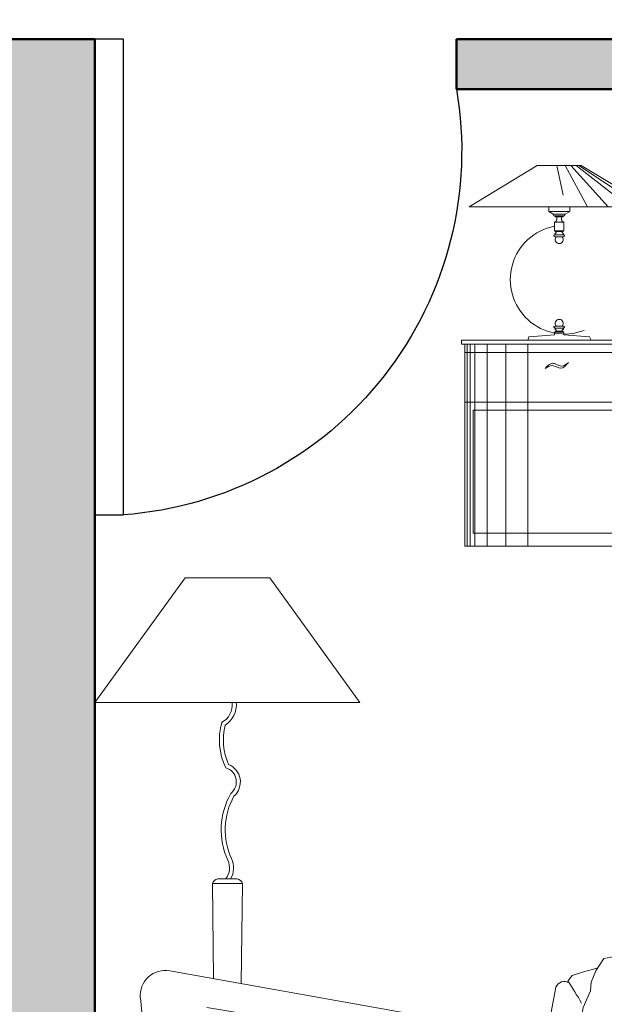
# Model space of a CAD drawing. Units: inches. Extents: x 1771 to 3025, y 319 to 889.
# Tile 27 of 35: x 2863 to 2921, y 521 to 619. Entities that reach past the tile are written whole.
import ezdxf

# ---------------------------------------------------------------- set-up
doc = ezdxf.new("R2010")
doc.units = ezdxf.units.IN
doc.header["$MEASUREMENT"] = 0
for name, color, linetype, lineweight in [('A-DOOR', 4, 'Continuous', 25), ('A-FURN', 8, 'Continuous', 18), ('A-WALL', 7, 'Continuous', 50), ('A-WALL-PATT', 254, 'Continuous', 13)]:
    doc.layers.add(name, color=color, linetype=linetype, lineweight=lineweight)

# ---------------------------------------------------------------- blocks, each defined once
blk = doc.blocks.new('A$C3908634B')
for p, q in [((184.3, 923.4), (19, 823.1)), ((237.5, 923.4), (184.3, 923.4)), ((190.2, 923.4), (237.5, 923.4)), ((231.9, 923.4), (247.3, 851.1)), ((284.7, 923.4), (237.5, 923.4)), ((237.5, 923.4), (290.6, 923.4)), ((251.7, 923.4), (305.7, 823.1)), ((266, 923.4), (356.4, 823.1)), ((278.7, 923.4), (406.8, 823.1)), ((284.7, 923.4), (436.3, 823.1)), ((290.6, 923.4), (456, 823.1)), ((237.5, 823.1), (19, 823.1)), ((212, 823.1), (212, 811.7)), ((237.5, 823.1), (456, 823.1)), ((263, 823.1), (263, 811.7)), ((212, 811.7), (223, 805.4)), ((212, 811.7), (237.5, 811.7)), ((223, 805.4), (224.6, 801.4)), ((223, 805.4), (237.5, 805.4)), ((250.4, 801.4), (224.6, 801.4)), ((226.9, 801.4), (228.3, 798.3)), ((228.3, 798.3), (237.5, 798.3)), ((228.3, 798.3), (231.3, 797.6)), ((231.1, 790.5), (230.2, 788)), ((231.5, 791.1), (231.1, 790.5)), ((231.3, 797.6), (232, 794.9)), ((231.6, 792.6), (231.5, 791.9)), ((231.5, 791.9), (231.5, 791.1)), ((231.9, 793.9), (231.6, 792.6)), ((232, 794.9), (231.9, 793.9)), ((263, 811.7), (237.5, 811.7)), ((252, 805.4), (237.5, 805.4)), ((246.7, 798.3), (237.5, 798.3)), ((243.7, 797.6), (243, 794.9)), ((243, 794.9), (243.1, 793.9)), ((243.1, 793.9), (243.4, 792.6)), ((243.4, 792.6), (243.4, 791.9)), ((243.4, 791.9), (243.4, 791.1)), ((243.4, 791.1), (243.9, 790.5)), ((246.7, 798.3), (243.7, 797.6)), ((243.9, 790.5), (244.8, 788)), ((248.1, 801.4), (246.7, 798.3)), ((252, 805.4), (250.4, 801.4)), ((263, 811.7), (252, 805.4)), ((227.8, 786.4), (226.2, 785.6)), ((226.2, 785.6), (226.2, 765)), ((226.2, 785.6), (248.8, 785.6)), ((226.2, 765), (227.6, 764.2)), ((226.2, 765), (237.5, 765)), ((227.6, 764.2), (228.5, 763.3)), ((230.2, 788), (227.8, 786.4)), ((248.8, 765), (237.5, 765)), ((244.8, 788), (247.2, 786.4)), ((247.4, 764.2), (246.5, 763.3)), ((247.2, 786.4), (248.8, 785.6)), ((248.8, 765), (247.4, 764.2)), ((248.8, 785.6), (248.8, 765)), ((224.8, 753.5), (224.7, 752.9)), ((224.7, 752.9), (224.8, 752.1)), ((225.3, 753.9), (224.8, 753.5)), ((224.8, 752.1), (225.2, 751.4)), ((225.2, 751.4), (225.6, 750.9)), ((225.7, 754.3), (225.3, 753.9)), ((225.6, 750.9), (228.1, 750.2)), ((226.3, 754.6), (225.7, 754.3)), ((227, 754.7), (226.3, 754.6)), ((227.9, 754.7), (227, 754.7)), ((227.4, 757.9), (227.1, 757.2)), ((227.1, 757.2), (227.3, 756.6)), ((227.3, 756.6), (227.8, 755.9)), ((227.7, 758.5), (227.4, 757.9)), ((228.6, 758.7), (227.7, 758.5)), ((227.8, 755.9), (228.9, 755.2)), ((228.9, 755.2), (227.9, 754.7)), ((228.1, 750.2), (229.9, 750)), ((228.5, 763.3), (229.4, 762.5)), ((228.5, 763.3), (237.5, 763.3)), ((229.4, 759.1), (228.6, 758.7)), ((228.9, 755.2), (237.5, 755.2)), ((229.4, 762.5), (230, 761.4)), ((229.8, 759.5), (229.4, 759.1)), ((230.1, 760.2), (229.8, 759.5)), ((229.9, 750), (232.4, 750.2)), ((230, 761.4), (230.1, 760.2)), ((232.4, 750.2), (237.5, 750.2)), ((246.5, 763.3), (237.5, 763.3)), ((246.1, 755.2), (237.5, 755.2)), ((242.6, 750.2), (237.5, 750.2)), ((245.1, 750), (242.6, 750.2)), ((245, 761.4), (244.9, 760.2)), ((244.9, 760.2), (245.2, 759.5)), ((245.6, 762.5), (245, 761.4)), ((246.9, 750.2), (245.1, 750)), ((245.2, 759.5), (245.6, 759.1)), ((246.5, 763.3), (245.6, 762.5)), ((245.6, 759.1), (246.4, 758.7)), ((247.2, 755.9), (246.1, 755.2)), ((246.1, 755.2), (247.1, 754.7)), ((246.4, 758.7), (247.3, 758.5)), ((249.4, 750.9), (246.9, 750.2)), ((247.1, 754.7), (248, 754.7)), ((247.7, 756.6), (247.2, 755.9)), ((247.3, 758.5), (247.6, 757.9)), ((247.6, 757.9), (247.9, 757.2)), ((247.9, 757.2), (247.7, 756.6)), ((248, 754.7), (248.7, 754.6)), ((248.7, 754.6), (249.3, 754.3)), ((249.3, 754.3), (249.7, 753.9)), ((249.8, 751.4), (249.4, 750.9)), ((249.7, 753.9), (250.2, 753.5)), ((250.2, 752.1), (249.8, 751.4)), ((250.2, 753.5), (250.3, 752.9)), ((250.3, 752.9), (250.2, 752.1)), ((224.7, 530.9), (224.8, 531.7)), ((224.8, 530.3), (224.7, 530.9)), ((224.8, 531.7), (225.2, 532.4)), ((225.3, 529.9), (224.8, 530.3)), ((225.2, 532.4), (225.6, 532.9)), ((225.7, 529.5), (225.3, 529.9)), ((225.6, 532.9), (228.1, 533.6)), ((226.3, 529.2), (225.7, 529.5)), ((227, 529.1), (226.3, 529.2)), ((227.9, 529.1), (227, 529.1)), ((227.1, 526.6), (227.3, 527.2)), ((227.4, 525.9), (227.1, 526.6)), ((227.3, 527.2), (227.8, 527.9)), ((227.7, 525.3), (227.4, 525.9)), ((228.6, 525.1), (227.7, 525.3)), ((227.8, 527.9), (228.9, 528.6)), ((228.9, 528.6), (227.9, 529.1)), ((228.1, 533.6), (229.9, 533.8)), ((228.9, 528.6), (237.5, 528.6)), ((230.3, 533.8), (237.5, 533.6)), ((242.6, 533.6), (237.5, 533.6)), ((246.1, 528.6), (237.5, 528.6)), ((245.1, 533.8), (242.6, 533.6)), ((246.9, 533.6), (245.1, 533.8)), ((246.1, 528.6), (247.1, 529.1)), ((247.2, 527.9), (246.1, 528.6)), ((246.4, 525.1), (247.3, 525.3)), ((249.4, 532.9), (246.9, 533.6)), ((247.1, 529.1), (248, 529.1)), ((247.7, 527.2), (247.2, 527.9)), ((247.3, 525.3), (247.6, 525.9)), ((247.6, 525.9), (247.9, 526.6)), ((247.9, 526.6), (247.7, 527.2)), ((248, 529.1), (248.7, 529.2)), ((248.7, 529.2), (249.3, 529.5)), ((249.3, 529.5), (249.7, 529.9)), ((249.8, 532.4), (249.4, 532.9)), ((249.7, 529.9), (250.2, 530.3)), ((250.2, 531.7), (249.8, 532.4)), ((250.3, 530.9), (250.2, 531.7)), ((250.2, 530.3), (250.3, 530.9)), ((164, 507.9), (161.1, 499.5)), ((164, 507.9), (226.2, 512.1)), ((226.2, 518.8), (227.6, 519.6)), ((226.2, 512.1), (226.2, 518.8)), ((226.2, 518.8), (237.5, 518.8)), ((227.6, 519.6), (228.5, 520.5)), ((228.5, 520.5), (229.4, 521.3)), ((229.4, 524.7), (228.6, 525.1)), ((229.8, 524.3), (229.4, 524.7)), ((229.4, 521.3), (230, 522.4)), ((229.4, 521.3), (237.5, 521.3)), ((230.1, 523.6), (229.8, 524.3)), ((230, 522.4), (230.1, 523.6)), ((245.6, 521.3), (237.5, 521.3)), ((248.8, 518.8), (237.5, 518.8)), ((244.9, 523.6), (245.2, 524.3)), ((245, 522.4), (244.9, 523.6)), ((245.6, 521.3), (245, 522.4)), ((245.2, 524.3), (245.6, 524.7)), ((245.6, 524.7), (246.4, 525.1)), ((246.5, 520.5), (245.6, 521.3)), ((247.4, 519.6), (246.5, 520.5)), ((248.8, 518.8), (247.4, 519.6)), ((248.8, 512.1), (248.8, 518.8)), ((311, 507.9), (248.8, 512.1)), ((311, 507.9), (315.3, 499.5)), ((475, 499.5), (0, 499.5)), ((0, 499.5), (0, 489.5)), ((475, 489.5), (0, 489.5)), ((8.7, 489.5), (8.7, 0)), ((14.1, 488.6), (14.1, 0)), ((21.3, 488.6), (21.3, 0)), ((33, 488.6), (33, 0)), ((62.7, 488.6), (62.7, 0)), ((107.6, 488.6), (107.6, 0)), ((161.1, 499.5), (237.5, 499.5)), ((161.6, 488.6), (161.6, 0)), ((315.3, 499.5), (237.5, 499.5)), ((467.1, 469.5), (8.7, 469.5)), ((467.1, 349.5), (8.7, 349.5)), ((28.7, 329.5), (28.7, 31.6)), ((447.1, 329.5), (28.7, 329.5)), ((28.7, 31.6), (447.1, 31.6)), ((8.7, 0), (467.1, 0))]:
    blk.add_line(p, q)
for centre, radius, start, end in [((250.5, 646.2), 131.8, 100.6234, 291.2), ((237.5, 743.5), 9.69, 137.7341, 270), ((237.5, 743.5), 9.69, 270, 42.2659), ((237.5, 540.3), 9.69, 90, 222.2659), ((237.5, 540.3), 9.69, 317.7341, 90)]:
    blk.add_arc(centre, radius, start, end)
for points, knots in [([(259.6, 445.5), (254.3, 441.1), (244.8, 433.2), (231.9, 440.9), (217, 446), (209.2, 437.1), (203.4, 430.5)], [0, 0, 0, 0, 18.381528, 32.980054, 40.875646, 63.595153, 63.595153, 63.595153, 63.595153]), ([(259.6, 445.5), (254, 438.6), (242.8, 424.9), (221, 442.9), (208.9, 434.4), (203.4, 430.5)], [0, 0, 0, 0, 22.772447, 45.052082, 63.466582, 63.466582, 63.466582, 63.466582])]:
    blk.add_open_spline(points, degree=3, knots=knots)
blk = doc.blocks.new('A$C0DCF6C46')
for p, q in [((179.4, 1650), (0, 1402.3)), ((179.4, 1650), (0, 1402.3)), ((179.4, 1650), (347.3, 1650)), ((179.4, 1650), (347.3, 1650)), ((347.3, 1650), (526.7, 1402.3)), ((347.3, 1650), (526.7, 1402.3)), ((0, 1402.3), (526.7, 1402.3)), ((0, 1402.3), (526.7, 1402.3)), ((1202.6, 1072.4), (1213.4, 1083.3)), ((1202.6, 1072.4), (1213.4, 1083.3)), ((1213.4, 1083.3), (1227.6, 1090.4)), ((1213.4, 1083.3), (1227.6, 1090.4)), ((1227.6, 1090.4), (1251, 1095.4)), ((1227.6, 1090.4), (1251, 1095.4)), ((1251, 1095.4), (1277.5, 1092)), ((1251, 1095.4), (1277.5, 1092)), ((1277.5, 1092), (1301.8, 1082.8)), ((1277.5, 1092), (1301.8, 1082.8)), ((1301.8, 1082.8), (1321.9, 1067.8)), ((1301.8, 1082.8), (1321.9, 1067.8)), ((1173.6, 1032.9), (1189.7, 1057.2)), ((1173.6, 1032.9), (1189.7, 1057.2)), ((1189.7, 1057.2), (1202.6, 1072.4)), ((1189.7, 1057.2), (1202.6, 1072.4)), ((1259.7, 1050.3), (1237.5, 1065.3)), ((1259.7, 1050.3), (1237.5, 1065.3)), ((1321.9, 1067.8), (1345.5, 1041.1)), ((1321.9, 1067.8), (1345.5, 1041.1)), ((233.4, 1042.3), (293.3, 1042.3)), ((233.4, 1042.3), (235.7, 853.7)), ((233.4, 1042.3), (293.3, 1042.3)), ((233.4, 1042.3), (235.7, 853.7)), ((244, 1051.7), (282.6, 1051.7)), ((244, 1051.7), (282.6, 1051.7)), ((293.3, 1042.3), (290.8, 843.9)), ((293.3, 1042.3), (290.8, 843.9)), ((1255.9, 1046.6), (1245.7, 1027.6)), ((1255.9, 1046.6), (1245.7, 1027.6)), ((1278.7, 1041.6), (1259.7, 1050.3)), ((1278.7, 1041.6), (1259.7, 1050.3)), ((1308.3, 1028.1), (1278.7, 1041.6)), ((1308.3, 1028.1), (1278.7, 1041.6)), ((1345.5, 1041.1), (1350.1, 1013.5)), ((1345.5, 1041.1), (1350.1, 1013.5)), ((1150.8, 970.5), (1173.6, 1032.9)), ((1150.8, 970.5), (1173.6, 1032.9)), ((1245.7, 1027.6), (1232.3, 1009.1)), ((1245.7, 1027.6), (1232.3, 1009.1)), ((1335.8, 1012.5), (1308.3, 1028.1)), ((1335.8, 1012.5), (1308.3, 1028.1)), ((1232.3, 1009.1), (1218.3, 983.7)), ((1232.3, 1009.1), (1218.3, 983.7)), ((1338.8, 997.1), (1335.8, 1012.5)), ((1338.8, 997.1), (1335.8, 1012.5)), ((1350.1, 1013.5), (1354.2, 991.7)), ((1350.1, 1013.5), (1354.2, 991.7)), ((1190.8, 987.7), (1188, 972.3)), ((1190.8, 987.7), (1188, 972.3)), ((1202.9, 975.4), (1190.8, 987.7)), ((1202.9, 975.4), (1190.8, 987.7)), ((1218.3, 983.7), (1202.9, 975.4)), ((1218.3, 983.7), (1202.9, 975.4)), ((1277.8, 994.4), (1265.6, 995)), ((1277.8, 994.4), (1265.6, 995)), ((1266, 980.7), (1284.6, 977.9)), ((1266, 980.7), (1284.6, 977.9)), ((1291.5, 983.2), (1277.8, 994.4)), ((1291.5, 983.2), (1277.8, 994.4)), ((1333.4, 980.2), (1324.9, 973.9)), ((1333.4, 980.2), (1324.9, 973.9)), ((1354.2, 991.7), (1333.4, 980.2)), ((1354.2, 991.7), (1333.4, 980.2)), ((1334, 990.3), (1338.8, 997.1)), ((1334, 990.3), (1338.8, 997.1)), ((1147.4, 942.9), (1150.8, 970.5)), ((1147.4, 942.9), (1150.8, 970.5)), ((1188, 972.3), (1182.6, 958)), ((1188, 972.3), (1182.6, 958)), ((1304.1, 966.6), (1297.6, 940.6)), ((1304.1, 966.6), (1297.6, 940.6)), ((1309.5, 977.7), (1304.1, 966.6)), ((1309.5, 977.7), (1304.1, 966.6)), ((1309.4, 969), (1312.6, 964.7)), ((1314.7, 968.9), (1309.4, 969)), ((1309.4, 969), (1312.6, 964.7)), ((1314.7, 968.9), (1309.4, 969)), ((1317.5, 977.7), (1309.5, 977.7)), ((1317.5, 977.7), (1309.5, 977.7)), ((1322.1, 963.3), (1318.8, 948.5)), ((1322.1, 963.3), (1318.8, 948.5)), ((1324.9, 973.9), (1322.1, 963.3)), ((1324.9, 973.9), (1322.1, 963.3)), ((1135.7, 928.2), (1147.4, 942.9)), ((1135.7, 928.2), (1147.4, 942.9)), ((1297.6, 940.6), (1286.8, 941.4)), ((1297.6, 940.6), (1286.8, 941.4)), ((1318.8, 948.5), (1307.6, 932.1)), ((1318.8, 948.5), (1307.6, 932.1)), ((1087.8, 908.4), (1135.7, 928.2)), ((1087.8, 908.4), (1135.7, 928.2)), ((1117, 920.9), (1113.7, 907.1)), ((1117, 920.9), (1113.7, 907.1)), ((1170.4, 917.1), (1156.8, 933.1)), ((1170.4, 917.1), (1156.8, 933.1)), ((1307.6, 932.1), (1282.5, 914.8)), ((1307.6, 932.1), (1282.5, 914.8)), ((1033.6, 897.7), (1060.7, 904.4)), ((1033.6, 897.7), (1060.7, 904.4)), ((1060.7, 904.4), (1087.8, 908.4)), ((1060.7, 904.4), (1087.8, 908.4)), ((1113.7, 907.1), (1121.7, 900.7)), ((1113.7, 907.1), (1121.7, 900.7)), ((1121.7, 900.7), (1119.4, 884.3)), ((1121.7, 900.7), (1119.4, 884.3)), ((1190.9, 864.1), (1144, 915.9)), ((1190.9, 864.1), (1144, 915.9)), ((1211.2, 886.7), (1170.4, 917.1)), ((1211.2, 886.7), (1170.4, 917.1)), ((1225.9, 897.6), (1208.3, 912.3)), ((1225.9, 897.6), (1208.3, 912.3)), ((1282.5, 914.8), (1267, 899.5)), ((1282.5, 914.8), (1267, 899.5)), ((1271.7, 895.8), (1295.1, 904.1)), ((1271.7, 895.8), (1295.1, 904.1)), ((1295.1, 904.1), (1310, 911.9)), ((1295.1, 904.1), (1310, 911.9)), ((1310, 911.9), (1334.4, 909.6)), ((1310, 911.9), (1334.4, 909.6)), ((1334.4, 909.6), (1359.2, 894.6)), ((1334.4, 909.6), (1359.2, 894.6)), ((995.7, 868.8), (1011.8, 893.6)), ((995.7, 868.8), (1011.8, 893.6)), ((1011.8, 893.6), (1033.6, 897.7)), ((1011.8, 893.6), (1033.6, 897.7)), ((1039.9, 891.8), (1050.5, 891.7)), ((1039.9, 891.8), (1050.5, 891.7)), ((1050.5, 891.7), (1058.4, 882.1)), ((1050.5, 891.7), (1058.4, 882.1)), ((1058.4, 882.1), (1076.1, 842.2)), ((1058.4, 882.1), (1076.1, 842.2)), ((1119.4, 884.3), (1119.3, 867.8)), ((1119.4, 884.3), (1119.3, 867.8)), ((1211.2, 886.7), (1190.9, 864.1)), ((1211.2, 886.7), (1190.9, 864.1)), ((1222.8, 881.9), (1223.6, 853.9)), ((1247, 848.8), (1222.8, 881.9)), ((1222.8, 881.9), (1223.6, 853.9)), ((1247, 848.8), (1222.8, 881.9)), ((1240.6, 890.8), (1225.9, 897.6)), ((1240.6, 890.8), (1225.9, 897.6)), ((1254.3, 890.2), (1240.6, 890.8)), ((1254.3, 890.2), (1240.6, 890.8)), ((1264.4, 895.9), (1254.3, 890.2)), ((1264.4, 895.9), (1254.3, 890.2)), ((1267, 899.5), (1271.7, 895.8)), ((1267, 899.5), (1271.7, 895.8)), ((1359.2, 894.6), (1384, 866.8)), ((1359.2, 894.6), (1384, 866.8)), ((148.7, 869.2), (799.3, 753.3)), ((148.7, 869.2), (799.3, 753.3)), ((986.5, 846.6), (995.7, 868.8)), ((986.5, 846.6), (995.7, 868.8)), ((1119.3, 867.8), (1135.5, 846.5)), ((1119.3, 867.8), (1135.5, 846.5)), ((1196.7, 865.6), (1204.6, 855)), ((1196.7, 865.6), (1204.6, 855)), ((1275.8, 869.8), (1284.7, 863.3)), ((1275.8, 869.8), (1284.7, 863.3)), ((1278.8, 848), (1280, 865.5)), ((1278.8, 848), (1280, 865.5)), ((1284.7, 863.3), (1296.3, 854.2)), ((1284.7, 863.3), (1296.3, 854.2)), ((1296.3, 854.2), (1303.8, 861.6)), ((1296.3, 854.2), (1303.8, 861.6)), ((1303.8, 861.6), (1313.5, 875.8)), ((1303.8, 861.6), (1313.5, 875.8)), ((1313.5, 875.8), (1318.8, 876.9)), ((1313.5, 875.8), (1318.8, 876.9)), ((1318.8, 876.9), (1321.4, 867.3)), ((1318.8, 876.9), (1321.4, 867.3)), ((1321.4, 867.3), (1342.5, 854.4)), ((1321.4, 867.3), (1342.5, 854.4)), ((1384, 866.8), (1396.6, 853.4)), ((1384, 866.8), (1396.6, 853.4)), ((984.8, 829.6), (986.5, 846.6)), ((984.8, 829.6), (986.5, 846.6)), ((1076.1, 842.2), (1077.8, 785.9)), ((1076.1, 842.2), (1077.8, 785.9)), ((1135.5, 846.5), (1162.3, 812.3)), ((1135.5, 846.5), (1162.3, 812.3)), ((1186.6, 860.4), (1212.2, 811.9)), ((1186.6, 860.4), (1212.2, 811.9)), ((1204.6, 855), (1219.4, 853.2)), ((1204.6, 855), (1219.4, 853.2)), ((1213.6, 851.7), (1221.1, 799.1)), ((1213.6, 851.7), (1221.1, 799.1)), ((1223.6, 853.9), (1255.4, 801.3)), ((1223.6, 853.9), (1255.4, 801.3)), ((1257.2, 799.9), (1247, 848.8)), ((1257.2, 799.9), (1247, 848.8)), ((1293.6, 844.7), (1278.8, 848)), ((1293.6, 844.7), (1278.8, 848)), ((1293.9, 818.2), (1293.6, 844.7)), ((1293.9, 818.2), (1293.6, 844.7)), ((1325.9, 840.7), (1312.2, 852)), ((1325.9, 840.7), (1312.2, 852)), ((1342.5, 854.4), (1362, 845.8)), ((1342.5, 854.4), (1362, 845.8)), ((1362, 845.8), (1365, 822.9)), ((1362, 845.8), (1365, 822.9)), ((1396.6, 853.4), (1411.8, 831)), ((1396.6, 853.4), (1411.8, 831)), ((1637.6, 846.8), (1643.1, 837.5)), ((1637.6, 846.8), (1643.1, 837.5)), ((915.2, 833), (897.4, 738.2)), ((915.2, 833), (897.4, 738.2)), ((970.2, 796.3), (984.8, 829.6)), ((970.2, 796.3), (984.8, 829.6)), ((1343.2, 816.2), (1325.9, 840.7)), ((1343.2, 816.2), (1325.9, 840.7)), ((1376.2, 822.8), (1365, 822.9)), ((1365, 822.9), (1371.3, 804.3)), ((1376.2, 822.8), (1365, 822.9)), ((1365, 822.9), (1371.3, 804.3)), ((1390.5, 825.9), (1376.2, 822.8)), ((1390.5, 825.9), (1376.2, 822.8)), ((1401.2, 832.2), (1390.5, 825.9)), ((1401.2, 832.2), (1390.5, 825.9)), ((1405.2, 808.3), (1401.2, 832.2)), ((1405.2, 808.3), (1401.2, 832.2)), ((1411.8, 831), (1422.3, 818.2)), ((1411.8, 831), (1422.3, 818.2)), ((1414.4, 832.1), (1447.5, 790.5)), ((1414.4, 832.1), (1447.5, 790.5)), ((1680.1, 723.7), (1660.3, 834.6)), ((1680.1, 723.7), (1660.3, 834.6)), ((167.7, 0), (90.2, 815.3)), ((167.7, 0), (90.2, 815.3)), ((1162.3, 812.3), (1187.5, 779.8)), ((1162.3, 812.3), (1187.5, 779.8)), ((1212.2, 811.9), (1236.7, 763.5)), ((1212.2, 811.9), (1236.7, 763.5)), ((1296.3, 781), (1293.9, 818.2)), ((1296.3, 781), (1293.9, 818.2)), ((1364.9, 799.6), (1343.2, 816.2)), ((1364.9, 799.6), (1343.2, 816.2)), ((1371.3, 804.3), (1380.5, 770.8)), ((1371.3, 804.3), (1380.5, 770.8)), ((1384, 803.7), (1372.4, 811.7)), ((1384, 803.7), (1372.4, 811.7)), ((1403.6, 803.5), (1384, 803.7)), ((1403.6, 803.5), (1384, 803.7)), ((1423.8, 807.1), (1403.6, 803.5)), ((1423.8, 807.1), (1403.6, 803.5)), ((1422.3, 818.2), (1423.8, 807.1)), ((1422.3, 818.2), (1423.8, 807.1)), ((821.8, 697.8), (222.3, 796.3)), ((821.8, 697.8), (222.3, 796.3)), ((966.3, 773.5), (970.2, 796.3)), ((966.3, 773.5), (970.2, 796.3)), ((1077.8, 785.9), (1071.1, 747.3)), ((1077.8, 785.9), (1071.1, 747.3)), ((1275.4, 760.5), (1257.2, 799.9)), ((1275.4, 760.5), (1257.2, 799.9)), ((1431.7, 801.7), (1440.8, 748.6)), ((1431.7, 801.7), (1440.8, 748.6)), ((1447.5, 790.5), (1463.6, 748.4)), ((1447.5, 790.5), (1463.6, 748.4)), ((963, 758.2), (966.3, 773.5)), ((963, 758.2), (966.3, 773.5)), ((1187.5, 779.8), (1212.2, 747.2)), ((1187.5, 779.8), (1212.2, 747.2)), ((1236.7, 763.5), (1253.3, 709.8)), ((1236.7, 763.5), (1253.3, 709.8)), ((1304.4, 731.6), (1296.3, 781)), ((1304.4, 731.6), (1296.3, 781)), ((1380.5, 770.8), (1387.2, 743.7)), ((1380.5, 770.8), (1387.2, 743.7)), ((965.8, 711), (963, 758.2)), ((965.8, 711), (963, 758.2)), ((1071.1, 747.3), (1070.3, 709.1)), ((1071.1, 747.3), (1070.3, 709.1)), ((1212.2, 747.2), (1239, 712)), ((1212.2, 747.2), (1239, 712)), ((1294.7, 714.7), (1275.4, 760.5)), ((1294.7, 714.7), (1275.4, 760.5)), ((1387.2, 743.7), (1387.1, 723)), ((1387.2, 743.7), (1387.1, 723)), ((1463.6, 748.4), (1467.1, 713.4)), ((1463.6, 748.4), (1467.1, 713.4)), ((816.5, 736.2), (823.2, 687.2)), ((816.5, 736.2), (823.2, 687.2)), ((1310.9, 687.6), (1304.4, 731.6)), ((1310.9, 687.6), (1304.4, 731.6)), ((949, 665.5), (965.8, 711)), ((949, 665.5), (965.8, 711)), ((1070.3, 709.1), (1067.4, 681)), ((1070.3, 709.1), (1067.4, 681)), ((1239, 712), (1250, 700.8)), ((1239, 712), (1250, 700.8)), ((1253.3, 709.8), (1262, 665.7)), ((1253.3, 709.8), (1262, 665.7)), ((1319.7, 657.3), (1294.7, 714.7)), ((1319.7, 657.3), (1294.7, 714.7)), ((1387.1, 723), (1385.3, 706.1)), ((1387.1, 723), (1385.3, 706.1)), ((1410.2, 693.1), (1433.6, 709.9)), ((1410.2, 693.1), (1433.6, 709.9)), ((1433.6, 709.9), (1459.6, 709.7)), ((1433.6, 709.9), (1459.6, 709.7)), ((1467.1, 713.4), (1510.5, 701.4)), ((1467.1, 713.4), (1510.5, 701.4)), ((823.2, 687.2), (840.7, 645.7)), ((823.2, 687.2), (840.7, 645.7)), ((919.8, 701.9), (919.8, 0)), ((919.8, 701.9), (919.8, 0)), ((1325.9, 701.8), (1321.2, 649.3)), ((1325.9, 701.8), (1321.2, 649.3)), ((1387.8, 675.8), (1325.9, 701.8)), ((1387.8, 675.8), (1325.9, 701.8)), ((1387.8, 675.8), (1410.2, 693.1)), ((1387.8, 675.8), (1410.2, 693.1)), ((1510.5, 701.4), (1562.3, 673.9)), ((1510.5, 701.4), (1562.3, 673.9)), ((1656.8, 701.9), (1656.8, 607.1)), ((1656.8, 701.9), (1656.8, 607.1)), ((816.1, 675.1), (831.6, 638.4)), ((816.1, 675.1), (831.6, 638.4)), ((952.4, 624.6), (949, 665.5)), ((952.4, 624.6), (949, 665.5)), ((968.1, 667.4), (995.8, 675.7)), ((968.1, 667.4), (995.8, 675.7)), ((995.8, 675.7), (1036.1, 673.3)), ((995.8, 675.7), (1036.1, 673.3)), ((1036.1, 673.3), (1074.2, 672.4)), ((1036.1, 673.3), (1074.2, 672.4)), ((1074.2, 672.4), (1099.7, 668.5)), ((1074.2, 672.4), (1099.7, 668.5)), ((1099.7, 668.5), (1130.9, 665.6)), ((1099.7, 668.5), (1130.9, 665.6)), ((1130.9, 665.6), (1156.4, 659.6)), ((1130.9, 665.6), (1156.4, 659.6)), ((1262, 665.7), (1274.2, 603)), ((1262, 665.7), (1274.2, 603)), ((1362.7, 657.4), (1387.8, 675.8)), ((1362.7, 657.4), (1387.8, 675.8)), ((1562.3, 673.9), (1616.6, 642.7)), ((1562.3, 673.9), (1616.6, 642.7)), ((840.7, 645.7), (862.6, 619.4)), ((840.7, 645.7), (862.6, 619.4)), ((1120.6, 625.4), (1130.3, 647.1)), ((1120.6, 625.4), (1130.3, 647.1)), ((1130.3, 647.1), (1138.8, 656.6)), ((1130.3, 647.1), (1138.8, 656.6)), ((1156.4, 659.6), (1194, 656.7)), ((1156.4, 659.6), (1194, 656.7)), ((1194, 656.7), (1230, 653.7)), ((1194, 656.7), (1230, 653.7)), ((1230, 653.7), (1248, 637.7)), ((1230, 653.7), (1248, 637.7)), ((1321.2, 649.3), (1340.1, 623.1)), ((1321.2, 649.3), (1340.1, 623.1)), ((1361.5, 647.4), (1329.7, 647.6)), ((1361.5, 647.4), (1329.7, 647.6)), ((1342.9, 632.7), (1362.7, 657.4)), ((1342.9, 632.7), (1362.7, 657.4)), ((1569.5, 644.7), (1548.9, 662.4)), ((1569.5, 644.7), (1548.9, 662.4)), ((831.6, 638.4), (853.4, 612.1)), ((831.6, 638.4), (853.4, 612.1)), ((1248, 637.7), (1261.6, 613.2)), ((1248, 637.7), (1261.6, 613.2)), ((1325.7, 613.7), (1342.9, 632.7)), ((1325.7, 613.7), (1342.9, 632.7)), ((1503.4, 603.8), (1505.1, 628.7)), ((1503.4, 603.8), (1505.1, 628.7)), ((1595.2, 618), (1569.5, 644.7)), ((1595.2, 618), (1569.5, 644.7)), ((1616.6, 642.7), (1655.6, 607.9)), ((1616.6, 642.7), (1655.6, 607.9)), ((853.4, 612.1), (858.7, 592.9)), ((853.4, 612.1), (858.7, 592.9)), ((862.6, 619.4), (867.8, 600.3)), ((862.6, 619.4), (867.8, 600.3)), ((961.2, 603.3), (952.4, 624.6)), ((961.2, 603.3), (952.4, 624.6)), ((1115.1, 607.9), (1115, 596.8)), ((1115.1, 607.9), (1115, 596.8)), ((1128.9, 611.5), (1115.1, 607.9)), ((1128.9, 611.5), (1115.1, 607.9)), ((1115.6, 599.4), (1119.9, 607.9)), ((1115.6, 599.4), (1119.9, 607.9)), ((1119.9, 607.9), (1120.6, 625.4)), ((1119.9, 607.9), (1120.6, 625.4)), ((1154.9, 605), (1128.9, 611.5)), ((1154.9, 605), (1128.9, 611.5)), ((1202.6, 606.7), (1154.9, 605)), ((1202.6, 606.7), (1154.9, 605)), ((1217.8, 581.7), (1202.6, 606.7)), ((1217.8, 581.7), (1202.6, 606.7)), ((1261.6, 613.2), (1259.1, 569.7)), ((1261.6, 613.2), (1259.1, 569.7)), ((1304.9, 592.7), (1325.7, 613.7)), ((1304.9, 592.7), (1325.7, 613.7)), ((1475.8, 608.8), (1478.2, 578)), ((1491.8, 546.1), (1475.8, 608.8)), ((1475.8, 608.8), (1478.2, 578)), ((1491.8, 546.1), (1475.8, 608.8)), ((1618.8, 582.8), (1595.2, 618)), ((1618.8, 582.8), (1595.2, 618)), ((1655.6, 607.9), (1695.2, 580.6)), ((1655.6, 607.9), (1695.2, 580.6)), ((867.8, 600.3), (810.7, 0)), ((867.8, 600.3), (810.7, 0)), ((858.7, 592.9), (816.6, 146.6)), ((858.7, 592.9), (816.6, 146.6)), ((994.1, 595.1), (961.2, 603.3)), ((994.1, 595.1), (961.2, 603.3)), ((1053.9, 576.6), (994.1, 595.1)), ((1053.9, 576.6), (994.1, 595.1)), ((1111.3, 595.2), (1113.2, 565.5)), ((1111.3, 595.2), (1113.2, 565.5)), ((1274.2, 603), (1280.6, 545.6)), ((1274.2, 603), (1280.6, 545.6)), ((1284.6, 575.8), (1304.9, 592.7)), ((1284.6, 575.8), (1304.9, 592.7)), ((1501, 578.9), (1503.4, 603.8)), ((1501, 578.9), (1503.4, 603.8)), ((1112.1, 561.3), (1053.9, 576.6)), ((1112.1, 561.3), (1053.9, 576.6)), ((1228.9, 581.6), (1217.8, 581.7)), ((1228.9, 581.6), (1217.8, 581.7)), ((1228.2, 558.8), (1228.9, 581.6)), ((1228.2, 558.8), (1228.9, 581.6)), ((1259.1, 569.7), (1252.7, 566)), ((1259.1, 569.7), (1252.7, 566)), ((1478.2, 578), (1493.9, 543.4)), ((1478.2, 578), (1493.9, 543.4)), ((1489.2, 562.6), (1501, 578.9)), ((1489.2, 562.6), (1501, 578.9)), ((1635.5, 547.1), (1618.8, 582.8)), ((1635.5, 547.1), (1618.8, 582.8)), ((1695.2, 580.6), (1732.1, 555.4)), ((1695.2, 580.6), (1732.1, 555.4)), ((1128.3, 528.3), (1112.1, 561.3)), ((1128.3, 528.3), (1112.1, 561.3)), ((1252.7, 566), (1228.2, 558.8)), ((1252.7, 566), (1228.2, 558.8)), ((1732.1, 555.4), (1753.8, 546.2)), ((1732.1, 555.4), (1753.8, 546.2)), ((1747.8, 525.5), (1746.4, 548.4)), ((1747.8, 525.5), (1746.4, 548.4)), ((1142.4, 502.7), (1128.3, 528.3)), ((1142.4, 502.7), (1128.3, 528.3)), ((1280.6, 545.6), (1294.5, 479.8)), ((1280.6, 545.6), (1294.5, 479.8)), ((1478.3, 517.6), (1491.8, 546.1)), ((1478.3, 517.6), (1491.8, 546.1)), ((1493.9, 543.4), (1527.3, 540.5)), ((1493.9, 543.4), (1527.3, 540.5)), ((1527.3, 540.5), (1578.2, 538)), ((1527.3, 540.5), (1578.2, 538)), ((1578.2, 538), (1610.5, 537.7)), ((1578.2, 538), (1610.5, 537.7)), ((1610.5, 537.7), (1634.4, 534.9)), ((1610.5, 537.7), (1634.4, 534.9)), ((1634.4, 534.9), (1652.2, 511.4)), ((1634.4, 534.9), (1652.2, 511.4)), ((1753.8, 546.2), (1776.6, 543.9)), ((1753.8, 546.2), (1776.6, 543.9)), ((1776.6, 543.9), (1784.6, 547)), ((1776.6, 543.9), (1784.6, 547)), ((1788.3, 543.8), (1777, 533.3)), ((1788.3, 543.8), (1777, 533.3)), ((1777, 533.3), (1777, 522.1)), ((1777, 533.3), (1777, 522.1)), ((1784.6, 547), (1807.3, 541.5)), ((1784.6, 547), (1807.3, 541.5)), ((1807.3, 541.5), (1836.4, 528.5)), ((1807.3, 541.5), (1836.4, 528.5)), ((1836.4, 528.5), (1857.6, 518.8)), ((1836.4, 528.5), (1857.6, 518.8)), ((1460.7, 501.8), (1478.3, 517.6)), ((1460.7, 501.8), (1478.3, 517.6)), ((1652.2, 511.4), (1671, 474.2)), ((1652.2, 511.4), (1671, 474.2)), ((1747.1, 502.7), (1747.8, 525.5)), ((1747.1, 502.7), (1747.8, 525.5)), ((1777, 522.1), (1776.8, 504.6)), ((1777, 522.1), (1776.8, 504.6)), ((1857.6, 518.8), (1884.1, 516)), ((1857.6, 518.8), (1884.1, 516)), ((1884.1, 516), (1912.1, 507.8)), ((1884.1, 516), (1912.1, 507.8)), ((1162.3, 464.9), (1142.4, 502.7)), ((1162.3, 464.9), (1142.4, 502.7)), ((1447.7, 477), (1460.7, 501.8)), ((1447.7, 477), (1460.7, 501.8)), ((1556.5, 478.8), (1575.3, 505.7)), ((1556.5, 478.8), (1575.3, 505.7)), ((1740, 481), (1747.1, 502.7)), ((1740, 481), (1747.1, 502.7)), ((1766.2, 498.3), (1749.2, 494.8)), ((1766.2, 498.3), (1749.2, 494.8)), ((1776.8, 504.6), (1766.2, 498.3)), ((1776.8, 504.6), (1766.2, 498.3)), ((1913, 492.4), (1906, 476.6)), ((1913, 492.4), (1906, 476.6)), ((1912.1, 507.8), (1913, 492.4)), ((1912.1, 507.8), (1913, 492.4)), ((1294.5, 479.8), (1303.6, 427.7)), ((1294.5, 479.8), (1303.6, 427.7)), ((1415.7, 451.8), (1447.7, 477)), ((1415.7, 451.8), (1447.7, 477)), ((1547.8, 455), (1556.5, 478.8)), ((1547.8, 455), (1556.5, 478.8)), ((1671, 474.2), (1681.4, 448.6)), ((1671, 474.2), (1681.4, 448.6)), ((1732.4, 458.3), (1740, 481)), ((1732.4, 458.3), (1740, 481)), ((1906, 476.6), (1884.1, 456)), ((1906, 476.6), (1884.1, 456)), ((1170.5, 433.5), (1162.3, 464.9)), ((1170.5, 433.5), (1162.3, 464.9)), ((1379, 432.4), (1415.7, 451.8)), ((1379, 432.4), (1415.7, 451.8)), ((1546.6, 431.1), (1547.8, 455)), ((1546.6, 431.1), (1547.8, 455)), ((1683.6, 450.7), (1697.6, 414)), ((1699.5, 448.5), (1683.6, 450.7)), ((1683.6, 450.7), (1697.6, 414)), ((1699.5, 448.5), (1683.6, 450.7)), ((1715.9, 452.6), (1699.5, 448.5)), ((1715.9, 452.6), (1699.5, 448.5)), ((1736.6, 455.1), (1715.9, 452.6)), ((1736.6, 455.1), (1715.9, 452.6)), ((1750.9, 447.5), (1736.6, 455.1)), ((1750.9, 447.5), (1736.6, 455.1)), ((1792.3, 453.6), (1780.1, 445.7)), ((1792.3, 453.6), (1780.1, 445.7)), ((1833.1, 442.1), (1792.3, 453.6)), ((1833.1, 442.1), (1792.3, 453.6)), ((1884.1, 456), (1859.1, 446.7)), ((1884.1, 456), (1859.1, 446.7)), ((1186.7, 397.9), (1170.5, 433.5)), ((1186.7, 397.9), (1170.5, 433.5)), ((1645.3, 444.1), (1649.7, 395.3)), ((1645.3, 444.1), (1649.7, 395.3)), ((1780.1, 445.7), (1750.9, 447.5)), ((1780.1, 445.7), (1750.9, 447.5)), ((1859.1, 446.7), (1833.1, 442.1)), ((1859.1, 446.7), (1833.1, 442.1)), ((862, 416.6), (851.4, 416.6)), ((862, 416.6), (851.4, 416.6)), ((1033.5, 416.6), (1544.9, 416.6)), ((1033.5, 416.6), (1544.9, 416.6)), ((1303.6, 427.7), (1308.2, 407)), ((1303.6, 427.7), (1308.2, 407)), ((1351.8, 416.7), (1315.1, 406.4)), ((1351.8, 416.7), (1315.1, 406.4)), ((1388.4, 423.3), (1351.8, 416.7)), ((1388.4, 423.3), (1351.8, 416.7)), ((1440.4, 418.1), (1388.4, 423.3)), ((1440.4, 418.1), (1388.4, 423.3)), ((1490.2, 415.6), (1440.4, 418.1)), ((1490.2, 415.6), (1440.4, 418.1)), ((1542.2, 420.5), (1490.2, 415.6)), ((1542.2, 420.5), (1490.2, 415.6)), ((1552.6, 389.1), (1542.2, 420.5)), ((1552.6, 389.1), (1542.2, 420.5)), ((1697.6, 414), (1703.2, 388)), ((1697.6, 414), (1703.2, 388)), ((882, 396.6), (866.1, 216.6)), ((882, 396.6), (866.1, 216.6)), ((1189.7, 380.9), (1186.7, 397.9)), ((1189.7, 380.9), (1186.7, 397.9)), ((1189.8, 391.5), (1189.7, 380.9)), ((1189.8, 391.5), (1189.7, 380.9)), ((1217.5, 406.6), (1189.8, 391.5)), ((1217.5, 406.6), (1189.8, 391.5)), ((1262, 404.2), (1217.5, 406.6)), ((1262, 404.2), (1217.5, 406.6)), ((1315.1, 406.4), (1262, 404.2)), ((1315.1, 406.4), (1262, 404.2)), ((1649.7, 395.3), (1660.1, 361.8)), ((1649.7, 395.3), (1660.1, 361.8)), ((1563, 357.2), (1552.6, 389.1)), ((1563, 357.2), (1552.6, 389.1)), ((1703.2, 388), (1711.8, 331.7)), ((1703.2, 388), (1711.8, 331.7)), ((1585.9, 307.2), (1563, 357.2)), ((1585.9, 307.2), (1563, 357.2)), ((1660.1, 361.8), (1662.9, 319.9)), ((1660.1, 361.8), (1662.9, 319.9)), ((1662.9, 319.9), (1645.5, 263.2)), ((1662.9, 319.9), (1645.5, 263.2)), ((1711.8, 331.7), (1721.8, 252.6)), ((1711.8, 331.7), (1721.8, 252.6)), ((1612.6, 261.4), (1585.9, 307.2)), ((1612.6, 261.4), (1585.9, 307.2)), ((1625.5, 214.1), (1612.6, 261.4)), ((1625.5, 214.1), (1612.6, 261.4)), ((1645.5, 263.2), (1632, 228.9)), ((1645.5, 263.2), (1632, 228.9)), ((1721.8, 252.6), (1729.7, 181.9)), ((1721.8, 252.6), (1729.7, 181.9)), ((846.1, 196.6), (829.9, 196.6)), ((846.1, 196.6), (829.9, 196.6)), ((1028.1, 196.6), (1544.2, 196.6)), ((1028.1, 196.6), (1544.2, 196.6)), ((1629.9, 164.2), (1625.5, 214.1)), ((1629.9, 164.2), (1625.5, 214.1)), ((1729.7, 181.9), (1734.7, 143.7)), ((1729.7, 181.9), (1734.7, 143.7)), ((825, 157.1), (152.8, 157.1)), ((825, 157.1), (152.8, 157.1)), ((989.7, 156.6), (1587.6, 156.6)), ((989.7, 156.6), (1587.6, 156.6)), ((1630.1, 127.6), (1629.9, 164.2)), ((1630.1, 127.6), (1629.9, 164.2)), ((825, 146.6), (153.8, 146.6)), ((825, 146.6), (153.8, 146.6)), ((243.8, 146.6), (221.9, 0)), ((243.8, 146.6), (221.9, 0)), ((244.6, 146.6), (245.3, 86.3)), ((244.6, 146.6), (245.3, 86.3)), ((282.1, 146.6), (281.3, 86.3)), ((282.1, 146.6), (281.3, 86.3)), ((746.4, 146.6), (768.4, 0)), ((746.4, 146.6), (768.4, 0)), ((989.7, 146.6), (1587.6, 146.6)), ((989.7, 146.6), (1587.6, 146.6)), ((1724.1, 142.7), (1698.1, 135)), ((1724.1, 142.7), (1698.1, 135)), ((1737.4, 151.1), (1724.1, 142.7)), ((1737.4, 151.1), (1724.1, 142.7)), ((1734.7, 143.7), (1737.8, 131)), ((1734.7, 143.7), (1737.8, 131)), ((1631, 102.1), (1630.1, 127.6)), ((1631, 102.1), (1630.1, 127.6)), ((1661.3, 116.7), (1650.2, 119.5)), ((1661.3, 116.7), (1650.2, 119.5)), ((1675.7, 123), (1661.3, 116.7)), ((1675.7, 123), (1661.3, 116.7)), ((1698.1, 135), (1675.7, 123)), ((1698.1, 135), (1675.7, 123)), ((1735.1, 122.5), (1717, 111.5)), ((1735.1, 122.5), (1717, 111.5)), ((1747.3, 126.1), (1735.1, 122.5)), ((1747.3, 126.1), (1735.1, 122.5)), ((1737.8, 131), (1747.9, 135.7)), ((1737.8, 131), (1747.9, 135.7)), ((1747.9, 135.7), (1755.6, 101.1)), ((1747.9, 135.7), (1755.6, 101.1)), ((236.8, 100), (245.2, 100)), ((236.8, 100), (245.2, 100)), ((1632.3, 70.8), (1631, 102.1)), ((1632.3, 70.8), (1631, 102.1)), ((1701, 106.3), (1675.6, 113.9)), ((1701, 106.3), (1675.6, 113.9)), ((1717, 111.5), (1701, 106.3)), ((1717, 111.5), (1701, 106.3)), ((1755.6, 101.1), (1777.7, 72.3)), ((1755.6, 101.1), (1777.7, 72.3)), ((234.6, 85), (244.2, 85)), ((234.6, 85), (244.2, 85)), ((245.3, 86.3), (281.3, 86.3)), ((245.3, 86.3), (281.3, 86.3)), ((239.8, 68.3), (239.8, 22.5)), ((239.8, 68.3), (286.9, 68.3)), ((239.8, 68.3), (239.8, 22.5)), ((239.8, 68.3), (286.9, 68.3)), ((286.9, 68.3), (286.9, 22.5)), ((286.9, 68.3), (286.9, 22.5)), ((1635.9, 52.2), (1632.3, 70.8)), ((1635.9, 52.2), (1632.3, 70.8)), ((1777.7, 72.3), (1806.8, 63.6)), ((1777.7, 72.3), (1806.8, 63.6)), ((1806.8, 63.6), (1841.7, 47.4)), ((1806.8, 63.6), (1841.7, 47.4)), ((1645.4, 43.1), (1635.9, 52.2)), ((1645.4, 43.1), (1635.9, 52.2)), ((1669.2, 38.7), (1645.4, 43.1)), ((1669.2, 38.7), (1645.4, 43.1)), ((1656.8, 41), (1656.8, 0)), ((1656.8, 41), (1656.8, 0)), ((1841.7, 47.4), (1849.6, 39.4)), ((1841.7, 47.4), (1849.6, 39.4)), ((1849.6, 39.4), (1849.4, 20.8)), ((1849.6, 39.4), (1849.4, 20.8)), ((116.8, 22.5), (116.8, 0)), ((116.8, 22.5), (165.6, 22.5)), ((116.8, 22.5), (116.8, 0)), ((116.8, 22.5), (165.6, 22.5)), ((225.2, 22.5), (409.9, 22.5)), ((225.2, 22.5), (409.9, 22.5)), ((409.9, 22.5), (409.9, 0)), ((409.9, 22.5), (409.9, 0)), ((1691.4, 35.3), (1669.2, 38.7)), ((1691.4, 35.3), (1669.2, 38.7)), ((1709, 35.2), (1691.4, 35.3)), ((1709, 35.2), (1691.4, 35.3)), ((1715.3, 26.6), (1709, 35.2)), ((1715.3, 26.6), (1709, 35.2)), ((1738, 13.7), (1715.3, 26.6)), ((1738, 13.7), (1715.3, 26.6)), ((1849.4, 20.8), (1824.4, 6.7)), ((1849.4, 20.8), (1824.4, 6.7)), ((1789.3, 2.7), (1738, 13.7)), ((1789.3, 2.7), (1738, 13.7)), ((1824.4, 6.7), (1789.3, 2.7)), ((1824.4, 6.7), (1789.3, 2.7)), ((116.8, 0), (409.9, 0)), ((116.8, 0), (409.9, 0)), ((919.8, 0), (937.1, 0)), ((919.8, 0), (937.1, 0)), ((1639.4, 0), (1656.8, 0)), ((1639.4, 0), (1656.8, 0))]:
    blk.add_line(p, q)
for centre, radius, start, end in [((232.2, 1398.2), 40.9, 298.591, 4.7801), ((232.2, 1398.2), 40.9, 298.591, 4.7801), ((232.2, 1398.2), 48.9, 302.7794, 4.7801), ((232.2, 1398.2), 48.9, 302.7794, 4.7801), ((374.6, 1328.2), 127.4, 164.5089, 205.7991), ((374.6, 1328.2), 127.4, 164.5089, 205.7991), ((374.6, 1328.2), 119.4, 166.0279, 204.234), ((374.6, 1328.2), 119.4, 166.0279, 204.234), ((251.6, 1244.5), 29.4, 308.7103, 73.8033), ((251.6, 1244.5), 29.4, 308.7103, 73.8033), ((251.6, 1244.5), 37.4, 311.1929, 67.9822), ((251.6, 1244.5), 37.4, 311.1929, 67.9822), ((395.6, 1149.4), 144.8, 150.115, 204.7751), ((395.6, 1149.4), 144.8, 150.115, 204.7751), ((395.6, 1149.4), 136.8, 150.7005, 204.7627), ((395.6, 1149.4), 136.8, 150.7005, 204.7627), ((231.9, 1073.6), 35.6, 321.9956, 25.2261), ((231.9, 1073.6), 35.6, 321.9956, 25.2261), ((231.9, 1073.6), 43.6, 329.6961, 25.182), ((231.9, 1073.6), 43.6, 329.6961, 25.182), ((246.1, 1038.6), 13.2, 98.8052, 163.9237), ((246.1, 1038.6), 13.2, 98.8052, 163.9237), ((280.6, 1038.6), 13.2, 16.0763, 81.1948), ((280.6, 1038.6), 13.2, 16.0763, 81.1948), ((1273.4, -169.1), 1079.2, 70.279, 86.636), ((1273.4, -169.1), 1079.2, 70.279, 86.636), ((139.9, 820), 50, 79.8912, 185.4337), ((139.9, 820), 50, 79.8912, 185.4337), ((1273.4, -169.1), 1079.2, 104.7019, 107.5271), ((1273.4, -169.1), 1079.2, 104.7019, 107.5271), ((933.1, 829.6), 18.2, 70.9411, 169.1012), ((933.1, 829.6), 18.2, 70.9411, 169.1012), ((1047.8, 778.9), 128.2, 140.7938, 148.0496), ((1047.8, 778.9), 128.2, 140.7938, 148.0496), ((241, 385.5), 838.8, 30.0042, 33.5227), ((241, 385.5), 838.8, 30.0042, 33.5227), ((2335, 385.5), 838.2, 146.5555, 159.4144), ((2335, 385.5), 838.2, 146.5555, 159.4144), ((1650.3, 825), 14.4, 42.1894, 120.2274), ((1650.3, 825), 14.4, 42.1894, 120.2274), ((796.6, 733.4), 20, 7.8584, 82.4843), ((796.6, 733.4), 20, 7.8584, 82.4843), ((929, 702.9), 43.5, 37.8135, 139.3209), ((929, 702.9), 43.5, 37.8135, 139.3209), ((1647.6, 702.9), 43.5, 45.0789, 176.3198), ((1647.6, 702.9), 43.5, 45.0789, 176.3198), ((923.6, 729.2), 27.6, 161.105, 262.178), ((923.6, 729.2), 27.6, 161.105, 262.178), ((929, 702.9), 33.5, 26.3854, 153.1276), ((929, 702.9), 33.5, 26.3854, 153.1276), ((1647.6, 702.9), 33.5, 26.8724, 191.3689), ((1647.6, 702.9), 33.5, 26.8724, 191.3689), ((1639.4, 689.8), 38.7, 155.7528, 188.1441), ((1639.4, 689.8), 38.7, 155.7528, 188.1441), ((1653, 729.2), 27.6, 277.822, 348.4179), ((1653, 729.2), 27.6, 277.822, 348.4179), ((2420.3, 406.7), 856.1, 160.2245, 163.3332), ((2420.3, 406.7), 856.1, 160.2245, 163.3332), ((2392.2, 407.9), 838, 160.7403, 162.7196), ((2392.2, 407.9), 838, 160.7403, 162.7196), ((156.3, 406.7), 856.1, 0.182, 12.766), ((156.3, 406.7), 856.1, 0.182, 12.766), ((176.7, 406.6), 845.7, 0.1617, 12.7147), ((176.7, 406.6), 845.7, 0.1617, 12.7147), ((241, 385.5), 838.8, 2.1238, 13.0913), ((241, 385.5), 838.8, 2.1238, 13.0913), ((862, 396.6), 20, 0, 90), ((862, 396.6), 20, 0, 90), ((1052.6, 376.5), 44.4, 115.3918, 154.207), ((1052.6, 376.5), 44.4, 115.3918, 154.207), ((178.3, 351), 836.1, 335.1756, 4.0003), ((178.3, 351), 836.1, 335.1756, 4.0003), ((2398.3, 351), 836.1, 179.4209, 204.8244), ((2398.3, 351), 836.1, 179.4209, 204.8244), ((846.1, 216.6), 20, 270, 0), ((846.1, 216.6), 20, 270, 0), ((1045.3, 237.5), 44.4, 202.0254, 247.0946), ((1045.3, 237.5), 44.4, 202.0254, 247.0946), ((1529.6, 238.5), 44.4, 289.1171, 341.8054), ((1529.6, 238.5), 44.4, 289.1171, 341.8054), ((262.7, 71.1), 23.1, 138.7741, 186.8798), ((262.7, 71.1), 23.1, 138.7741, 186.8798), ((263.9, 71.1), 23.1, 353.1202, 41.2259), ((263.9, 71.1), 23.1, 353.1202, 41.2259)]:
    blk.add_arc(centre, radius, start, end)
blk = doc.blocks.new('A$C4223307F')
blk.add_line((768.4, 0), (810.7, 0))
blk.add_blockref('A$C0DCF6C46', (0, 0))
blk = doc.blocks.new('A$C061F63B6')
blk.add_blockref('A$C4223307F', (0, 0))
blk = doc.blocks.new('DOOR-36B')
blk.add_lwpolyline([(0, 47.366), (2.836, 47.366), (2.836, 0), (0, 0)], close=True)
blk.add_arc((0.178, 11.122), 36.341, 350.30151, 85.80589)

msp = doc.modelspace()

# ---------------------------------------------------------------- hatches: boundary and pattern name
at = {"layer": 'A-WALL-PATT'}
h = msp.add_hatch(color=256, dxfattribs=at)
h.dxf.hatch_style = 1
h.paths.add_polyline_path([(2870.685, 879.484), (2892.728, 879.484), (2892.728, 889.484), (2842.685, 889.484), (2842.685, 879.484), (2865.685, 879.484), (2865.685, 831.484), (2870.685, 831.484)])
h.paths.add_polyline_path([(2983.637, 889.484), (2940.728, 889.484), (2940.728, 879.484), (2961.685, 879.484), (2961.685, 795.484), (2865.685, 795.484), (2865.685, 759.484), (2865.685, 665.484), (2870.685, 665.484), (2870.685, 712.85), (2870.685, 790.484), (2978.685, 790.484), (2978.685, 795.484), (2966.685, 795.484), (2966.685, 879.484), (2983.637, 879.484)])
h.paths.add_polyline_path([(3024.685, 889.484), (3001.637, 889.484), (3001.637, 879.484), (3014.685, 879.484), (3014.685, 790.484), (3014.685, 769.459), (3024.685, 769.459)])
h.paths.add_polyline_path([(3024.685, 721.459), (3014.685, 721.459), (3014.685, 670.484), (2906.685, 670.484), (2906.685, 665.484), (2925.685, 665.484), (2925.685, 653.484), (2930.685, 653.484), (2930.685, 665.484), (3014.685, 665.484), (3014.685, 650.024), (3024.685, 650.024)])
h.paths.add_polyline_path([(3024.685, 632.024), (3014.685, 632.024), (3014.685, 617.484), (2925.685, 617.484), (2906.685, 617.484), (2906.685, 612.484), (3014.685, 612.484), (3014.685, 581.957), (3024.685, 581.957)])
h.paths.add_polyline_path([(3024.685, 533.957), (3014.685, 533.957), (3014.685, 480.484), (2870.685, 480.484), (2870.685, 617.484), (2860.685, 617.484), (2860.685, 544.484), (2769.685, 544.484), (2769.685, 534.484), (2860.685, 534.484), (2860.685, 470.484), (3014.685, 470.484), (3014.685, 453.613), (3024.685, 453.613)])
h.paths.add_polyline_path([(3024.685, 405.613), (3014.685, 405.613), (3014.685, 394.484), (2860.685, 394.484), (2860.685, 384.484), (3024.685, 384.484)])
h.paths.add_polyline_path([(2733.685, 643.435), (2723.685, 643.435), (2723.685, 534.484), (2733.685, 534.484)])
h.paths.add_polyline_path([(2733.685, 754.484), (2829.685, 754.484), (2829.685, 759.484), (2733.685, 759.484), (2733.685, 843.439, -0.008336), (2732.382, 843.484), (2723.685, 843.484), (2723.685, 691.435), (2733.685, 691.435)])
h.paths.add_polyline_path([(2794.685, 889.484), (2723.685, 889.484), (2723.685, 879.484), (2794.685, 879.484)])

# ---------------------------------------------------------------- linework, layer by layer
at = {"layer": 'A-WALL'}
for p, q in [((2870.685, 617.484), (2860.685, 617.484)), ((2870.685, 617.484), (2870.685, 480.484)), ((2925.685, 617.484), (2906.685, 617.484)), ((2906.685, 617.484), (2906.685, 612.484)), ((3014.685, 612.484), (2906.685, 612.484))]:
    msp.add_line(p, q, dxfattribs=at)

# ---------------------------------------------------------------- block references
at = {"layer": 'A-DOOR', "extrusion": (0, 0, -1), "zscale": -1, "rotation": 180}
msp.add_blockref('DOOR-36B', (-2870.685, 617.484), dxfattribs=at)
at = {"layer": 'A-FURN'}
for name, p, xscale, yscale, zscale in [('A$C3908634B', (2907.17, 567.009), 0.0410441893854556, 0.0410441893854556, 0.0410441893854556), ('A$C061F63B6', (2870.685, 481.196), 0.0500958271542837, 0.0500958271542837, 0.0500958271542837)]:
    msp.add_blockref(name, p, dxfattribs=dict(at, xscale=xscale, yscale=yscale, zscale=zscale))

doc.saveas('drawing.dxf')
